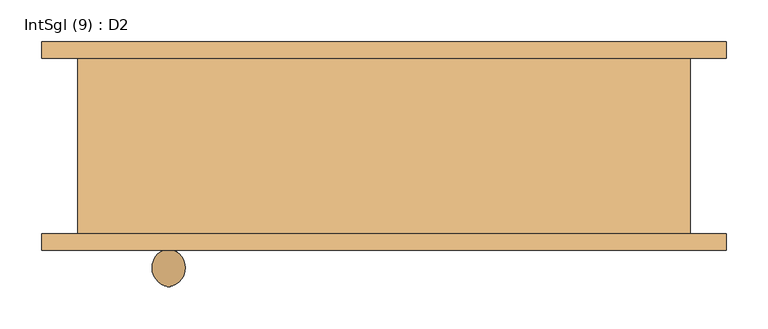
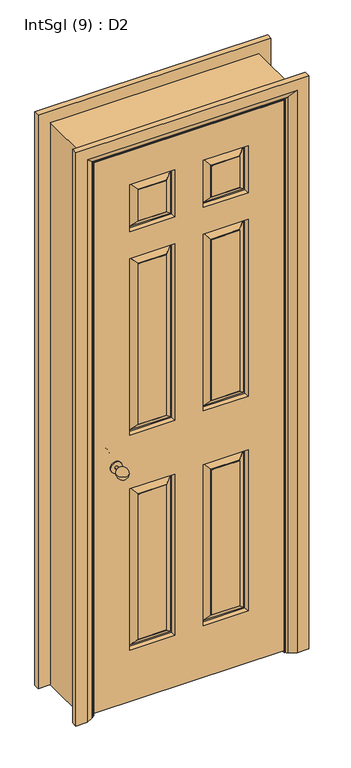
"""IFC4 building model written with IfcOpenShell, lengths in millimetres: door geometry, IntSgl (9) : D2."""

from ifc_helpers import new_model, si_unit, point, frame, origin, place, context, project, spatial, polyline, circle_curve, ellipse_curve, trimmed, outline, extrude, faceted_brep, source, transform, mapped, element, save
from ifc_brep_helpers import plane_surface, cylinder_surface, revolved_surface, advanced_brep


def intsgl_9_d2_d16f3bbe(model_context):
    return source(origin(), model_context, "Body", "SolidModel", [
        advanced_brep(
        [(-253.0, -48.0, 900.0), (-263.0, -48.0, 900.0), (-258.0, -3.562589, 900.0), (-253.0, -63.0, 900.0), (-263.0, -63.0, 900.0), (-278.0, -67.0, 900.0), (-238.0, -67.0, 900.0), (-278.0, -63.0, 900.0), (-238.0, -63.0, 900.0)],
        [
            (0, 1, circle_curve(frame((-258.0, -48.0, 900.0), z_axis=(0.0, 1.0, 0.0), x_axis=(-1.0, 0.0, 0.0)), 5.0)),
            (1, 2, circle_curve(frame((-254.8115138, -26.4213505, 900.0), z_axis=(0.0, 0.0, -1.0), x_axis=(0.0, -1.0, 0.0)), 23.0800654)),
            (2, 0, circle_curve(frame((-261.1884862, -26.4213505, 900.0), z_axis=(0.0, 0.0, -1.0), x_axis=(0.0, -1.0, 0.0)), 23.0800654)),
            (1, 0, circle_curve(frame((-258.0, -48.0, 900.0), z_axis=(0.0, 1.0, 0.0), x_axis=(-1.0, 0.0, 0.0)), 5.0)),
            (0, 3),
            (3, 4, circle_curve(frame((-258.0, -63.0, 900.0), z_axis=(0.0, 1.0, 0.0), x_axis=(-1.0, 0.0, 0.0)), 5.0)),
            (4, 1),
            (4, 3, circle_curve(frame((-258.0, -63.0, 900.0), z_axis=(0.0, 1.0, 0.0), x_axis=(-1.0, 0.0, 0.0)), 5.0)),
            (5, 6, circle_curve(frame((-258.0, -67.0, 900.0), z_axis=(0.0, -1.0, 0.0), x_axis=(1.0, 0.0, 0.0)), 20.0)),
            (6, 5, circle_curve(frame((-258.0, -67.0, 900.0), z_axis=(0.0, -1.0, 0.0), x_axis=(1.0, 0.0, 0.0)), 20.0)),
            (7, 8, circle_curve(frame((-258.0, -63.0, 900.0), z_axis=(0.0, 1.0, 0.0), x_axis=(1.0, 0.0, 0.0)), 20.0)),
            (8, 7, circle_curve(frame((-258.0, -63.0, 900.0), z_axis=(0.0, 1.0, 0.0), x_axis=(1.0, 0.0, 0.0)), 20.0)),
            (5, 7),
            (8, 6),
        ],
        [
            revolved_surface(trimmed(ellipse_curve(frame((-254.8115138, -26.4213505, 900.0), z_axis=(0.0, 0.0, 1.0), x_axis=(0.0, -1.0, 0.0)), 23.0800654, 23.0800654), [point((-258.0, -3.562589, 900.0))], [point((-263.0, -48.0, 900.0))], True, "CARTESIAN"), (-258.0, -63.0, 900.0), (0.0, -1.0, 0.0)),
            cylinder_surface(frame((-258.0, -63.0, 900.0), z_axis=(0.0, -1.0, 0.0), x_axis=(-1.0, 0.0, 0.0)), 5.0),
            plane_surface(frame((-238.0, -67.0, 900.0), z_axis=(0.0, -1.0, 0.0), x_axis=(0.0, 0.0, 1.0))),
            plane_surface(frame((-238.0, -63.0, 900.0), z_axis=(0.0, 1.0, 0.0), x_axis=(0.0, 0.0, -1.0))),
            cylinder_surface(frame((-258.0, -63.0, 900.0), z_axis=(0.0, -1.0, 0.0), x_axis=(1.0, 0.0, 0.0)), 20.0),
        ],
        [
            (0, [[1, 2, 3]]),
            (0, [[-2, 4, -3]]),
            (1, [[-1, 5, 6, 7]]),
            (1, [[-4, -7, 8, -5]]),
            (2, [[9, 10]]),
            (3, [[11, 12], [-6, -8]]),
            (4, [[-9, 13, -12, 14]]),
            (4, [[-10, -14, -11, -13]]),
        ],
    ),
        advanced_brep(
        [(-253.0, -124.0, 900.0), (-258.0, -168.437411, 900.0), (-263.0, -124.0, 900.0), (-263.0, -109.0, 900.0), (-253.0, -109.0, 900.0), (-278.0, -105.0, 900.0), (-238.0, -105.0, 900.0), (-278.0, -109.0, 900.0), (-238.0, -109.0, 900.0)],
        [
            (0, 1, circle_curve(frame((-261.1884862, -145.5786495, 900.0), z_axis=(0.0, 0.0, -1.0), x_axis=(0.0, 1.0, 0.0)), 23.0800654)),
            (1, 2, circle_curve(frame((-254.8115138, -145.5786495, 900.0), z_axis=(0.0, 0.0, -1.0), x_axis=(0.0, 1.0, 0.0)), 23.0800654)),
            (2, 0, circle_curve(frame((-258.0, -124.0, 900.0), z_axis=(0.0, -1.0, 0.0), x_axis=(-1.0, 0.0, 0.0)), 5.0)),
            (0, 2, circle_curve(frame((-258.0, -124.0, 900.0), z_axis=(0.0, -1.0, 0.0), x_axis=(-1.0, 0.0, 0.0)), 5.0)),
            (2, 3),
            (3, 4, circle_curve(frame((-258.0, -109.0, 900.0), z_axis=(0.0, -1.0, 0.0), x_axis=(-1.0, 0.0, 0.0)), 5.0)),
            (4, 0),
            (4, 3, circle_curve(frame((-258.0, -109.0, 900.0), z_axis=(0.0, -1.0, 0.0), x_axis=(-1.0, 0.0, 0.0)), 5.0)),
            (5, 6, circle_curve(frame((-258.0, -105.0, 900.0), z_axis=(0.0, 1.0, 0.0), x_axis=(1.0, 0.0, 0.0)), 20.0)),
            (6, 5, circle_curve(frame((-258.0, -105.0, 900.0), z_axis=(0.0, 1.0, 0.0), x_axis=(1.0, 0.0, 0.0)), 20.0)),
            (7, 8, circle_curve(frame((-258.0, -109.0, 900.0), z_axis=(0.0, -1.0, 0.0), x_axis=(1.0, 0.0, 0.0)), 20.0)),
            (8, 7, circle_curve(frame((-258.0, -109.0, 900.0), z_axis=(0.0, -1.0, 0.0), x_axis=(1.0, 0.0, 0.0)), 20.0)),
            (6, 8),
            (7, 5),
        ],
        [
            revolved_surface(trimmed(ellipse_curve(frame((-254.8115138, -145.5786495, 900.0), z_axis=(0.0, 0.0, -1.0), x_axis=(0.0, 1.0, 0.0)), 23.0800654, 23.0800654), [point((-258.0, -168.437411, 900.0))], [point((-263.0, -124.0, 900.0))], True, "CARTESIAN"), (-258.0, -109.0, 900.0), (0.0, 1.0, 0.0)),
            cylinder_surface(frame((-258.0, -109.0, 900.0), z_axis=(0.0, 1.0, 0.0), x_axis=(-1.0, 0.0, 0.0)), 5.0),
            plane_surface(frame((-238.0, -105.0, 900.0), z_axis=(0.0, 1.0, 0.0), x_axis=(0.0, 0.0, 1.0))),
            plane_surface(frame((-238.0, -109.0, 900.0), z_axis=(0.0, -1.0, 0.0), x_axis=(0.0, 0.0, -1.0))),
            cylinder_surface(frame((-258.0, -109.0, 900.0), z_axis=(0.0, 1.0, 0.0), x_axis=(1.0, 0.0, 0.0)), 20.0),
        ],
        [
            (0, [[1, 2, 3]]),
            (0, [[-1, 4, -2]]),
            (1, [[5, 6, 7, -3]]),
            (1, [[-7, 8, -5, -4]]),
            (2, [[9, 10]]),
            (3, [[11, 12], [-8, -6]]),
            (4, [[13, -11, 14, -10]]),
            (4, [[-14, -12, -13, -9]]),
        ],
    ),
        faceted_brep([(-333.0, -67.0, 2058.0), (333.0, -67.0, 2058.0), (333.0, -67.0, 8.0), (-333.0, -67.0, 8.0), (-50.0, -67.0, 800.0), (-208.0, -67.0, 800.0), (-208.0, -67.0, 200.0), (-50.0, -67.0, 200.0), (208.0, -67.0, 800.0), (50.0, -67.0, 800.0), (50.0, -67.0, 200.0), (208.0, -67.0, 200.0), (-50.0, -67.0, 1658.0), (-208.0, -67.0, 1658.0), (-208.0, -67.0, 1000.0), (-50.0, -67.0, 1000.0), (208.0, -67.0, 1658.0), (50.0, -67.0, 1658.0), (50.0, -67.0, 1000.0), (208.0, -67.0, 1000.0), (-50.0, -67.0, 1933.0), (-208.0, -67.0, 1933.0), (-208.0, -67.0, 1758.0), (-50.0, -67.0, 1758.0), (208.0, -67.0, 1933.0), (50.0, -67.0, 1933.0), (50.0, -67.0, 1758.0), (208.0, -67.0, 1758.0), (-80.0, -67.0, 230.0), (-178.0, -67.0, 230.0), (-178.0, -67.0, 770.0), (-80.0, -67.0, 770.0), (178.0, -67.0, 230.0), (80.0, -67.0, 230.0), (80.0, -67.0, 770.0), (178.0, -67.0, 770.0), (-80.0, -67.0, 1030.0), (-178.0, -67.0, 1030.0), (-178.0, -67.0, 1628.0), (-80.0, -67.0, 1628.0), (178.0, -67.0, 1030.0), (80.0, -67.0, 1030.0), (80.0, -67.0, 1628.0), (178.0, -67.0, 1628.0), (-80.0, -67.0, 1788.0), (-178.0, -67.0, 1788.0), (-178.0, -67.0, 1903.0), (-80.0, -67.0, 1903.0), (178.0, -67.0, 1788.0), (80.0, -67.0, 1788.0), (80.0, -67.0, 1903.0), (178.0, -67.0, 1903.0), (-333.0, -105.0, 2058.0), (-333.0, -105.0, 8.0), (333.0, -105.0, 8.0), (333.0, -105.0, 2058.0), (50.0, -105.0, 800.0), (208.0, -105.0, 800.0), (208.0, -105.0, 200.0), (50.0, -105.0, 200.0), (-208.0, -105.0, 800.0), (-50.0, -105.0, 800.0), (-50.0, -105.0, 200.0), (-208.0, -105.0, 200.0), (50.0, -105.0, 1658.0), (208.0, -105.0, 1658.0), (208.0, -105.0, 1000.0), (50.0, -105.0, 1000.0), (-208.0, -105.0, 1658.0), (-50.0, -105.0, 1658.0), (-50.0, -105.0, 1000.0), (-208.0, -105.0, 1000.0), (50.0, -105.0, 1933.0), (208.0, -105.0, 1933.0), (208.0, -105.0, 1758.0), (50.0, -105.0, 1758.0), (-208.0, -105.0, 1933.0), (-50.0, -105.0, 1933.0), (-50.0, -105.0, 1758.0), (-208.0, -105.0, 1758.0), (80.0, -105.0, 230.0), (178.0, -105.0, 230.0), (178.0, -105.0, 770.0), (80.0, -105.0, 770.0), (-178.0, -105.0, 230.0), (-80.0, -105.0, 230.0), (-80.0, -105.0, 770.0), (-178.0, -105.0, 770.0), (80.0, -105.0, 1030.0), (178.0, -105.0, 1030.0), (178.0, -105.0, 1628.0), (80.0, -105.0, 1628.0), (-178.0, -105.0, 1030.0), (-80.0, -105.0, 1030.0), (-80.0, -105.0, 1628.0), (-178.0, -105.0, 1628.0), (80.0, -105.0, 1788.0), (178.0, -105.0, 1788.0), (178.0, -105.0, 1903.0), (80.0, -105.0, 1903.0), (-178.0, -105.0, 1788.0), (-80.0, -105.0, 1788.0), (-80.0, -105.0, 1903.0), (-178.0, -105.0, 1903.0), (80.0, -104.0, 230.0), (80.0, -104.0, 770.0), (58.0, -90.0, 208.0), (78.0, -104.0, 228.0), (78.0, -104.0, 772.0), (58.0, -90.0, 792.0), (53.0, -90.0, 203.0), (53.0, -90.0, 797.0), (178.0, -104.0, 770.0), (180.0, -104.0, 772.0), (200.0, -90.0, 792.0), (205.0, -90.0, 797.0), (178.0, -104.0, 230.0), (180.0, -104.0, 228.0), (200.0, -90.0, 208.0), (205.0, -90.0, 203.0), (-178.0, -104.0, 230.0), (-178.0, -104.0, 770.0), (-200.0, -90.0, 208.0), (-180.0, -104.0, 228.0), (-180.0, -104.0, 772.0), (-200.0, -90.0, 792.0), (-205.0, -90.0, 203.0), (-205.0, -90.0, 797.0), (-80.0, -104.0, 770.0), (-78.0, -104.0, 772.0), (-58.0, -90.0, 792.0), (-53.0, -90.0, 797.0), (-80.0, -104.0, 230.0), (-78.0, -104.0, 228.0), (-58.0, -90.0, 208.0), (-53.0, -90.0, 203.0), (80.0, -104.0, 1030.0), (80.0, -104.0, 1628.0), (58.0, -90.0, 1008.0), (78.0, -104.0, 1028.0), (78.0, -104.0, 1630.0), (58.0, -90.0, 1650.0), (53.0, -90.0, 1003.0), (53.0, -90.0, 1655.0), (178.0, -104.0, 1628.0), (180.0, -104.0, 1630.0), (200.0, -90.0, 1650.0), (205.0, -90.0, 1655.0), (178.0, -104.0, 1030.0), (180.0, -104.0, 1028.0), (200.0, -90.0, 1008.0), (205.0, -90.0, 1003.0), (-178.0, -104.0, 1030.0), (-178.0, -104.0, 1628.0), (-200.0, -90.0, 1008.0), (-180.0, -104.0, 1028.0), (-180.0, -104.0, 1630.0), (-200.0, -90.0, 1650.0), (-205.0, -90.0, 1003.0), (-205.0, -90.0, 1655.0), (-80.0, -104.0, 1628.0), (-78.0, -104.0, 1630.0), (-58.0, -90.0, 1650.0), (-53.0, -90.0, 1655.0), (-80.0, -104.0, 1030.0), (-78.0, -104.0, 1028.0), (-58.0, -90.0, 1008.0), (-53.0, -90.0, 1003.0), (80.0, -104.0, 1788.0), (80.0, -104.0, 1903.0), (58.0, -90.0, 1766.0), (78.0, -104.0, 1786.0), (78.0, -104.0, 1905.0), (58.0, -90.0, 1925.0), (53.0, -90.0, 1761.0), (53.0, -90.0, 1930.0), (178.0, -104.0, 1903.0), (180.0, -104.0, 1905.0), (200.0, -90.0, 1925.0), (205.0, -90.0, 1930.0), (178.0, -104.0, 1788.0), (180.0, -104.0, 1786.0), (200.0, -90.0, 1766.0), (205.0, -90.0, 1761.0), (-178.0, -104.0, 1788.0), (-178.0, -104.0, 1903.0), (-200.0, -90.0, 1766.0), (-180.0, -104.0, 1786.0), (-180.0, -104.0, 1905.0), (-200.0, -90.0, 1925.0), (-205.0, -90.0, 1761.0), (-205.0, -90.0, 1930.0), (-80.0, -104.0, 1903.0), (-78.0, -104.0, 1905.0), (-58.0, -90.0, 1925.0), (-53.0, -90.0, 1930.0), (-80.0, -104.0, 1788.0), (-78.0, -104.0, 1786.0), (-58.0, -90.0, 1766.0), (-53.0, -90.0, 1761.0), (-80.0, -68.0, 230.0), (-80.0, -68.0, 770.0), (-58.0, -82.0, 208.0), (-78.0, -68.0, 228.0), (-78.0, -68.0, 772.0), (-58.0, -82.0, 792.0), (-53.0, -82.0, 203.0), (-53.0, -82.0, 797.0), (-178.0, -68.0, 770.0), (-180.0, -68.0, 772.0), (-200.0, -82.0, 792.0), (-205.0, -82.0, 797.0), (-178.0, -68.0, 230.0), (-180.0, -68.0, 228.0), (-200.0, -82.0, 208.0), (-205.0, -82.0, 203.0), (178.0, -68.0, 230.0), (178.0, -68.0, 770.0), (200.0, -82.0, 208.0), (180.0, -68.0, 228.0), (180.0, -68.0, 772.0), (200.0, -82.0, 792.0), (205.0, -82.0, 203.0), (205.0, -82.0, 797.0), (80.0, -68.0, 770.0), (78.0, -68.0, 772.0), (58.0, -82.0, 792.0), (53.0, -82.0, 797.0), (80.0, -68.0, 230.0), (78.0, -68.0, 228.0), (58.0, -82.0, 208.0), (53.0, -82.0, 203.0), (-80.0, -68.0, 1030.0), (-80.0, -68.0, 1628.0), (-58.0, -82.0, 1008.0), (-78.0, -68.0, 1028.0), (-78.0, -68.0, 1630.0), (-58.0, -82.0, 1650.0), (-53.0, -82.0, 1003.0), (-53.0, -82.0, 1655.0), (-178.0, -68.0, 1628.0), (-180.0, -68.0, 1630.0), (-200.0, -82.0, 1650.0), (-205.0, -82.0, 1655.0), (-178.0, -68.0, 1030.0), (-180.0, -68.0, 1028.0), (-200.0, -82.0, 1008.0), (-205.0, -82.0, 1003.0), (178.0, -68.0, 1030.0), (178.0, -68.0, 1628.0), (200.0, -82.0, 1008.0), (180.0, -68.0, 1028.0), (180.0, -68.0, 1630.0), (200.0, -82.0, 1650.0), (205.0, -82.0, 1003.0), (205.0, -82.0, 1655.0), (80.0, -68.0, 1628.0), (78.0, -68.0, 1630.0), (58.0, -82.0, 1650.0), (53.0, -82.0, 1655.0), (80.0, -68.0, 1030.0), (78.0, -68.0, 1028.0), (58.0, -82.0, 1008.0), (53.0, -82.0, 1003.0), (-80.0, -68.0, 1788.0), (-80.0, -68.0, 1903.0), (-58.0, -82.0, 1766.0), (-78.0, -68.0, 1786.0), (-78.0, -68.0, 1905.0), (-58.0, -82.0, 1925.0), (-53.0, -82.0, 1761.0), (-53.0, -82.0, 1930.0), (-178.0, -68.0, 1903.0), (-180.0, -68.0, 1905.0), (-200.0, -82.0, 1925.0), (-205.0, -82.0, 1930.0), (-178.0, -68.0, 1788.0), (-180.0, -68.0, 1786.0), (-200.0, -82.0, 1766.0), (-205.0, -82.0, 1761.0), (178.0, -68.0, 1788.0), (178.0, -68.0, 1903.0), (200.0, -82.0, 1766.0), (180.0, -68.0, 1786.0), (180.0, -68.0, 1905.0), (200.0, -82.0, 1925.0), (205.0, -82.0, 1761.0), (205.0, -82.0, 1930.0), (80.0, -68.0, 1903.0), (78.0, -68.0, 1905.0), (58.0, -82.0, 1925.0), (53.0, -82.0, 1930.0), (80.0, -68.0, 1788.0), (78.0, -68.0, 1786.0), (58.0, -82.0, 1766.0), (53.0, -82.0, 1761.0)], [[[0, 1, 2, 3], [4, 5, 6, 7], [8, 9, 10, 11], [12, 13, 14, 15], [16, 17, 18, 19], [20, 21, 22, 23], [24, 25, 26, 27]], [[28, 29, 30, 31]], [[32, 33, 34, 35]], [[36, 37, 38, 39]], [[40, 41, 42, 43]], [[44, 45, 46, 47]], [[48, 49, 50, 51]], [[52, 53, 54, 55], [56, 57, 58, 59], [60, 61, 62, 63], [64, 65, 66, 67], [68, 69, 70, 71], [72, 73, 74, 75], [76, 77, 78, 79]], [[80, 81, 82, 83]], [[84, 85, 86, 87]], [[88, 89, 90, 91]], [[92, 93, 94, 95]], [[96, 97, 98, 99]], [[100, 101, 102, 103]], [[3, 53, 52, 0]], [[2, 54, 53, 3]], [[1, 55, 54, 2]], [[0, 52, 55, 1]], [[104, 80, 83, 105]], [[106, 107, 108, 109]], [[56, 59, 110, 111]], [[83, 82, 112, 105]], [[108, 113, 114, 109]], [[111, 115, 57, 56]], [[82, 81, 116, 112]], [[113, 117, 118, 114]], [[115, 119, 58, 57]], [[104, 116, 81, 80]], [[107, 117, 113, 108], [105, 112, 116, 104]], [[106, 118, 117, 107]], [[110, 119, 115, 111], [109, 114, 118, 106]], [[59, 58, 119, 110]], [[120, 84, 87, 121]], [[122, 123, 124, 125]], [[60, 63, 126, 127]], [[87, 86, 128, 121]], [[124, 129, 130, 125]], [[127, 131, 61, 60]], [[86, 85, 132, 128]], [[129, 133, 134, 130]], [[131, 135, 62, 61]], [[120, 132, 85, 84]], [[123, 133, 129, 124], [121, 128, 132, 120]], [[122, 134, 133, 123]], [[126, 135, 131, 127], [125, 130, 134, 122]], [[63, 62, 135, 126]], [[136, 88, 91, 137]], [[138, 139, 140, 141]], [[64, 67, 142, 143]], [[91, 90, 144, 137]], [[140, 145, 146, 141]], [[143, 147, 65, 64]], [[90, 89, 148, 144]], [[145, 149, 150, 146]], [[147, 151, 66, 65]], [[136, 148, 89, 88]], [[139, 149, 145, 140], [137, 144, 148, 136]], [[138, 150, 149, 139]], [[142, 151, 147, 143], [141, 146, 150, 138]], [[67, 66, 151, 142]], [[152, 92, 95, 153]], [[154, 155, 156, 157]], [[68, 71, 158, 159]], [[95, 94, 160, 153]], [[156, 161, 162, 157]], [[159, 163, 69, 68]], [[94, 93, 164, 160]], [[161, 165, 166, 162]], [[163, 167, 70, 69]], [[152, 164, 93, 92]], [[155, 165, 161, 156], [153, 160, 164, 152]], [[154, 166, 165, 155]], [[158, 167, 163, 159], [157, 162, 166, 154]], [[71, 70, 167, 158]], [[168, 96, 99, 169]], [[170, 171, 172, 173]], [[72, 75, 174, 175]], [[99, 98, 176, 169]], [[172, 177, 178, 173]], [[175, 179, 73, 72]], [[98, 97, 180, 176]], [[177, 181, 182, 178]], [[179, 183, 74, 73]], [[168, 180, 97, 96]], [[171, 181, 177, 172], [169, 176, 180, 168]], [[170, 182, 181, 171]], [[174, 183, 179, 175], [173, 178, 182, 170]], [[75, 74, 183, 174]], [[184, 100, 103, 185]], [[186, 187, 188, 189]], [[76, 79, 190, 191]], [[103, 102, 192, 185]], [[188, 193, 194, 189]], [[191, 195, 77, 76]], [[102, 101, 196, 192]], [[193, 197, 198, 194]], [[195, 199, 78, 77]], [[184, 196, 101, 100]], [[187, 197, 193, 188], [185, 192, 196, 184]], [[186, 198, 197, 187]], [[190, 199, 195, 191], [189, 194, 198, 186]], [[79, 78, 199, 190]], [[200, 28, 31, 201]], [[202, 203, 204, 205]], [[4, 7, 206, 207]], [[31, 30, 208, 201]], [[204, 209, 210, 205]], [[207, 211, 5, 4]], [[30, 29, 212, 208]], [[209, 213, 214, 210]], [[211, 215, 6, 5]], [[200, 212, 29, 28]], [[203, 213, 209, 204], [201, 208, 212, 200]], [[202, 214, 213, 203]], [[206, 215, 211, 207], [205, 210, 214, 202]], [[7, 6, 215, 206]], [[216, 32, 35, 217]], [[218, 219, 220, 221]], [[8, 11, 222, 223]], [[35, 34, 224, 217]], [[220, 225, 226, 221]], [[223, 227, 9, 8]], [[34, 33, 228, 224]], [[225, 229, 230, 226]], [[227, 231, 10, 9]], [[216, 228, 33, 32]], [[219, 229, 225, 220], [217, 224, 228, 216]], [[218, 230, 229, 219]], [[222, 231, 227, 223], [221, 226, 230, 218]], [[11, 10, 231, 222]], [[232, 36, 39, 233]], [[234, 235, 236, 237]], [[12, 15, 238, 239]], [[39, 38, 240, 233]], [[236, 241, 242, 237]], [[239, 243, 13, 12]], [[38, 37, 244, 240]], [[241, 245, 246, 242]], [[243, 247, 14, 13]], [[232, 244, 37, 36]], [[235, 245, 241, 236], [233, 240, 244, 232]], [[234, 246, 245, 235]], [[238, 247, 243, 239], [237, 242, 246, 234]], [[15, 14, 247, 238]], [[248, 40, 43, 249]], [[250, 251, 252, 253]], [[16, 19, 254, 255]], [[43, 42, 256, 249]], [[252, 257, 258, 253]], [[255, 259, 17, 16]], [[42, 41, 260, 256]], [[257, 261, 262, 258]], [[259, 263, 18, 17]], [[248, 260, 41, 40]], [[251, 261, 257, 252], [249, 256, 260, 248]], [[250, 262, 261, 251]], [[254, 263, 259, 255], [253, 258, 262, 250]], [[19, 18, 263, 254]], [[264, 44, 47, 265]], [[266, 267, 268, 269]], [[20, 23, 270, 271]], [[47, 46, 272, 265]], [[268, 273, 274, 269]], [[271, 275, 21, 20]], [[46, 45, 276, 272]], [[273, 277, 278, 274]], [[275, 279, 22, 21]], [[264, 276, 45, 44]], [[267, 277, 273, 268], [265, 272, 276, 264]], [[266, 278, 277, 267]], [[270, 279, 275, 271], [269, 274, 278, 266]], [[23, 22, 279, 270]], [[280, 48, 51, 281]], [[282, 283, 284, 285]], [[24, 27, 286, 287]], [[51, 50, 288, 281]], [[284, 289, 290, 285]], [[287, 291, 25, 24]], [[50, 49, 292, 288]], [[289, 293, 294, 290]], [[291, 295, 26, 25]], [[280, 292, 49, 48]], [[283, 293, 289, 284], [281, 288, 292, 280]], [[282, 294, 293, 283]], [[286, 295, 291, 287], [285, 290, 294, 282]], [[27, 26, 295, 286]]]),
        faceted_brep([(-335.0, -105.0, 0.0), (-367.0, -105.0, 0.0), (-367.0, 105.0, 0.0), (-335.0, 105.0, 0.0), (-335.0, 105.0, 2060.0), (-335.0, -105.0, 2060.0), (-367.0, 105.0, 2092.0), (-367.0, -105.0, 2092.0), (335.0, -105.0, 0.0), (335.0, 105.0, 0.0), (367.0, 105.0, 0.0), (367.0, -105.0, 0.0), (335.0, -105.0, 2060.0), (367.0, -105.0, 2092.0), (367.0, 105.0, 2092.0), (335.0, 105.0, 2060.0)], [[[0, 1, 2, 3]], [[3, 4, 5, 0]], [[2, 6, 4, 3]], [[1, 7, 6, 2]], [[0, 5, 7, 1]], [[8, 9, 10, 11]], [[12, 8, 11, 13]], [[13, 11, 10, 14]], [[14, 10, 9, 15]], [[15, 9, 8, 12]], [[4, 15, 12, 5]], [[6, 14, 15, 4]], [[7, 13, 14, 6]], [[5, 12, 13, 7]]]),
        extrude(outline(polyline([(0.0, -316.0), (2041.0, -316.0), (2041.0, 316.0), (0.0, 316.0), (0.0, 335.0), (2060.0, 335.0), (2060.0, -335.0), (0.0, -335.0), (0.0, -316.0)])), frame((0.0, -65.0, 0.0), z_axis=(0.0, 1.0, 0.0), x_axis=(0.0, 0.0, 1.0)), (0.0, 0.0, 1.0), 32.0),
        advanced_brep(
        [(-410.0, 125.0, 0.0), (-370.0, 125.0, 0.0), (-344.0, 111.0, 0.0), (-340.0, 105.0, 0.0), (-410.0, 105.0, 0.0), (-410.0, 105.0, 2135.0), (-410.0, 125.0, 2135.0), (-340.0, 105.0, 2065.0), (340.0, 105.0, 2065.0), (340.0, 105.0, 0.0), (410.0, 105.0, 0.0), (410.0, 105.0, 2135.0), (-344.0, 111.0, 2069.0), (-370.0, 125.0, 2095.0), (410.0, 125.0, 2135.0), (410.0, 125.0, 0.0), (370.0, 125.0, 0.0), (370.0, 125.0, 2095.0), (344.0, 111.0, 0.0), (344.0, 111.0, 2069.0)],
        [
            (0, 1),
            (1, 2),
            (2, 3, circle_curve(frame((-348.0, 104.0, 0.0), z_axis=(0.0, 0.0, -1.0), x_axis=(-1.0, 0.0, 0.0)), 8.0622577)),
            (3, 4),
            (4, 0),
            (4, 5),
            (5, 6),
            (6, 0),
            (3, 7),
            (7, 8),
            (8, 9),
            (9, 10),
            (10, 11),
            (11, 5),
            (2, 12),
            (12, 7, ellipse_curve(frame((-348.0, 104.0, 2073.0), z_axis=(-0.7071067811865475, 0.0, -0.7071067811865475), x_axis=(0.7071067811865474, 0.0, -0.7071067811865476)), 11.4017543, 8.0622577)),
            (1, 13),
            (13, 12),
            (6, 14),
            (14, 15),
            (15, 16),
            (16, 17),
            (17, 13),
            (10, 15),
            (14, 11),
            (9, 18, circle_curve(frame((348.0, 104.0, 0.0), z_axis=(0.0, 0.0, -1.0), x_axis=(1.0, 0.0, 0.0)), 8.0622577)),
            (18, 16),
            (19, 18),
            (8, 19, ellipse_curve(frame((348.0, 104.0, 2073.0), z_axis=(0.7071067811865475, 0.0, -0.7071067811865475), x_axis=(0.7071067811865474, 0.0, 0.7071067811865476)), 11.4017543, 8.0622577)),
            (19, 17),
            (12, 19),
        ],
        [
            plane_surface(frame((-340.0, 105.0, 0.0), z_axis=(0.0, 0.0, -1.0), x_axis=(0.0, 1.0, 0.0))),
            plane_surface(frame((-410.0, 125.0, 0.0), z_axis=(-1.0, 0.0, 0.0), x_axis=(0.0, 0.0, 1.0))),
            plane_surface(frame((-410.0, 105.0, 0.0), z_axis=(0.0, -1.0, 0.0), x_axis=(0.0, 0.0, 1.0))),
            cylinder_surface(frame((-348.0, 104.0, 0.0), z_axis=(0.0, 0.0, -1.0), x_axis=(-1.0, 0.0, 0.0)), 8.0622577),
            plane_surface(frame((-344.0, 111.0, 0.0), z_axis=(0.4740998230350183, 0.8804710999221749, 0.0), x_axis=(0.0, 0.0, 1.0))),
            plane_surface(frame((-370.0, 125.0, 0.0), z_axis=(0.0, 1.0, 0.0), x_axis=(0.0, 0.0, 1.0))),
            plane_surface(frame((410.0, 125.0, 2135.0), z_axis=(1.0, 0.0, 0.0), x_axis=(0.0, 0.0, -1.0))),
            plane_surface(frame((340.0, 105.0, 0.0), z_axis=(0.0, 0.0, -1.0), x_axis=(0.0, 1.0, 0.0))),
            cylinder_surface(frame((348.0, 104.0, 2065.0), z_axis=(0.0, 0.0, 1.0), x_axis=(1.0, 0.0, 0.0)), 8.0622577),
            plane_surface(frame((344.0, 111.0, 2069.0), z_axis=(-0.4740998230350183, 0.8804710999221749, 0.0), x_axis=(0.0, 0.0, -1.0))),
            plane_surface(frame((-410.0, 125.0, 2135.0), z_axis=(0.0, 0.0, 1.0), x_axis=(1.0, 0.0, 0.0))),
            cylinder_surface(frame((-340.0, 104.0, 2073.0), z_axis=(-1.0, 0.0, 0.0), x_axis=(0.0, 0.0, 1.0)), 8.0622577),
            plane_surface(frame((-344.0, 111.0, 2069.0), z_axis=(0.0, 0.8804710999221749, -0.4740998230350183), x_axis=(1.0, 0.0, 0.0))),
        ],
        [
            (0, [[1, 2, 3, 4, 5]]),
            (1, [[6, 7, 8, -5]]),
            (2, [[9, 10, 11, 12, 13, 14, -6, -4]]),
            (3, [[15, 16, -9, -3]]),
            (4, [[17, 18, -15, -2]]),
            (5, [[-8, 19, 20, 21, 22, 23, -17, -1]]),
            (6, [[-13, 24, -20, 25]]),
            (7, [[-24, -12, 26, 27, -21]]),
            (8, [[28, -26, -11, 29]]),
            (9, [[-22, -27, -28, 30]]),
            (10, [[-14, -25, -19, -7]]),
            (11, [[31, -29, -10, -16]]),
            (12, [[-23, -30, -31, -18]]),
        ],
    ),
        advanced_brep(
        [(410.0, -125.0, 0.0), (370.0, -125.0, 0.0), (344.0, -111.0, 0.0), (340.0, -105.0, 0.0), (410.0, -105.0, 0.0), (410.0, -105.0, 2135.0), (410.0, -125.0, 2135.0), (340.0, -105.0, 2065.0), (-340.0, -105.0, 2065.0), (-340.0, -105.0, 0.0), (-410.0, -105.0, 0.0), (-410.0, -105.0, 2135.0), (344.0, -111.0, 2069.0), (370.0, -125.0, 2095.0), (-410.0, -125.0, 2135.0), (-410.0, -125.0, 0.0), (-370.0, -125.0, 0.0), (-370.0, -125.0, 2095.0), (-344.0, -111.0, 0.0), (-344.0, -111.0, 2069.0)],
        [
            (0, 1),
            (1, 2),
            (2, 3, circle_curve(frame((348.0, -104.0, 0.0), z_axis=(0.0, 0.0, -1.0), x_axis=(1.0, 0.0, 0.0)), 8.0622577)),
            (3, 4),
            (4, 0),
            (4, 5),
            (5, 6),
            (6, 0),
            (3, 7),
            (7, 8),
            (8, 9),
            (9, 10),
            (10, 11),
            (11, 5),
            (2, 12),
            (12, 7, ellipse_curve(frame((348.0, -104.0, 2073.0), z_axis=(0.7071067811865475, 0.0, -0.7071067811865475), x_axis=(-0.7071067811865474, 0.0, -0.7071067811865476)), 11.4017543, 8.0622577)),
            (1, 13),
            (13, 12),
            (6, 14),
            (14, 15),
            (15, 16),
            (16, 17),
            (17, 13),
            (10, 15),
            (14, 11),
            (9, 18, circle_curve(frame((-348.0, -104.0, 0.0), z_axis=(0.0, 0.0, -1.0), x_axis=(-1.0, 0.0, 0.0)), 8.0622577)),
            (18, 16),
            (19, 18),
            (8, 19, ellipse_curve(frame((-348.0, -104.0, 2073.0), z_axis=(-0.7071067811865475, 0.0, -0.7071067811865475), x_axis=(-0.7071067811865474, 0.0, 0.7071067811865476)), 11.4017543, 8.0622577)),
            (19, 17),
            (12, 19),
        ],
        [
            plane_surface(frame((340.0, -105.0, 0.0), z_axis=(0.0, 0.0, -1.0), x_axis=(0.0, -1.0, 0.0))),
            plane_surface(frame((410.0, -125.0, 0.0), z_axis=(1.0, 0.0, 0.0), x_axis=(0.0, 0.0, 1.0))),
            plane_surface(frame((410.0, -105.0, 0.0), z_axis=(0.0, 1.0, 0.0), x_axis=(0.0, 0.0, 1.0))),
            cylinder_surface(frame((348.0, -104.0, 0.0), z_axis=(0.0, 0.0, -1.0), x_axis=(1.0, 0.0, 0.0)), 8.0622577),
            plane_surface(frame((344.0, -111.0, 0.0), z_axis=(-0.4740998230350183, -0.8804710999221749, 0.0), x_axis=(0.0, 0.0, 1.0))),
            plane_surface(frame((370.0, -125.0, 0.0), z_axis=(0.0, -1.0, 0.0), x_axis=(0.0, 0.0, 1.0))),
            plane_surface(frame((-410.0, -125.0, 2135.0), z_axis=(-1.0, 0.0, 0.0), x_axis=(0.0, 0.0, -1.0))),
            plane_surface(frame((-340.0, -105.0, 0.0), z_axis=(0.0, 0.0, -1.0), x_axis=(0.0, -1.0, 0.0))),
            cylinder_surface(frame((-348.0, -104.0, 2065.0), z_axis=(0.0, 0.0, 1.0), x_axis=(-1.0, 0.0, 0.0)), 8.0622577),
            plane_surface(frame((-344.0, -111.0, 2069.0), z_axis=(0.4740998230350183, -0.8804710999221749, 0.0), x_axis=(0.0, 0.0, -1.0))),
            plane_surface(frame((410.0, -125.0, 2135.0), z_axis=(0.0, 0.0, 1.0), x_axis=(-1.0, 0.0, 0.0))),
            cylinder_surface(frame((340.0, -104.0, 2073.0), z_axis=(1.0, 0.0, 0.0), x_axis=(0.0, 0.0, 1.0)), 8.0622577),
            plane_surface(frame((344.0, -111.0, 2069.0), z_axis=(0.0, -0.8804710999221749, -0.4740998230350183), x_axis=(-1.0, 0.0, 0.0))),
        ],
        [
            (0, [[1, 2, 3, 4, 5]]),
            (1, [[6, 7, 8, -5]]),
            (2, [[9, 10, 11, 12, 13, 14, -6, -4]]),
            (3, [[15, 16, -9, -3]]),
            (4, [[17, 18, -15, -2]]),
            (5, [[-8, 19, 20, 21, 22, 23, -17, -1]]),
            (6, [[-13, 24, -20, 25]]),
            (7, [[-24, -12, 26, 27, -21]]),
            (8, [[28, -26, -11, 29]]),
            (9, [[-22, -27, -28, 30]]),
            (10, [[-14, -25, -19, -7]]),
            (11, [[31, -29, -10, -16]]),
            (12, [[-23, -30, -31, -18]]),
        ],
    ),
    ])


if __name__ == "__main__":
    model = new_model("IFC4")
    model_context = context("Model", 3, world=origin())
    ifc_project = project(units=[si_unit("LENGTHUNIT", "METRE", prefix="MILLI")], contexts=[model_context])
    site = spatial("IfcSite", under=ifc_project)
    building = spatial("IfcBuilding", under=site)
    placement = place(None, origin())
    intsgl_9_d2_shape = intsgl_9_d2_d16f3bbe(model_context)
    element("IfcDoor", 1, ObjectType="IntSgl (9) : D2", at=placement, inside=building, context=model_context, shape_type="MappedRepresentation", body=[
        mapped(intsgl_9_d2_shape, transform((0.0, 0.0, 0.0), x_axis=(1.0, 0.0, 0.0), y_axis=(0.0, 1.0, 0.0), z_axis=(0.0, 0.0, 1.0))),
    ])
    save(model, "model.ifc")

# Revit data of these elements
# Type "IntSgl (9) : D2"
#   Type Mark = "50"
#   Operation = "SingleSwingRight"
#   Manufacturer = "Revit"
#   Keynote = "L20"
#   UnderCut = 8 mm
#   Tolerance = 2 mm
#   Thickness = 38 mm
#   Structural Tolerance = 8 mm
#   StopDepth = 32 mm
#   Stop Thickness = 19 mm
#   Stile Top Rail = 125 mm
#   Stile Shutting = 125 mm
#   Stile Muntin Rail = 100 mm
#   Stile Lock Rail = 200 mm
#   Stile Intermediate/Frieze = 100 mm
#   Stile Hanging = 125 mm
#   Stile Bottom Rail = 200 mm
#   Rough Width = 750 mm
#   Rough Height = 2100 mm
#   Height to Top Lock Rail = 1000 mm
#   Handle Z Distance = 900 mm
#   Handle X Distance = 75 mm
#   Frame Thickness = 32 mm
#   Door Panel Width = 666 mm
#   Height = 2100 mm
#   Width = 750 mm
#   Door Panel Thickness = 38 mm
#   Door Panel Offset = 0 mm
#   Door Panel Height = 2050 mm
#   Architrave Setback = 5 mm
#   Vis - Ironmongery = yes
#   Material Ironmongery = Door - Handle
#   Material Frame = Door - Frame/Mullion
#   Material Door = Door - Panel
#   Material Architrave = Door - Architrave
#   Function = (empty or 0)
#   Wall Closure = (empty or 0)
# Element 1 (IfcDoor, "IntSgl (9) : D2")
#   Materials on its faces: "Door - Panel", "Door - Architrave", "Door - Frame/Mullion", "Door - Handle"
# Materials
#   "Door - Handle": colour RGB 0 0 0, transparency 0, Keynote = "P21", Cost = 0, Export to IFC = 0
#   "Door - Frame/Mullion": class "Wood", colour RGB 212 179 113, transparency 0, Keynote = "L20", Cost = 0, Export to IFC = 0
#   "Door - Panel": class "Wood", colour RGB 210 159 95, transparency 0, Keynote = "L20", Cost = 0, Export to IFC = 0
#   "Door - Architrave": class "Wood", colour RGB 154 90 5, transparency 0, Keynote = "P20", Cost = 0, Export to IFC = 0
